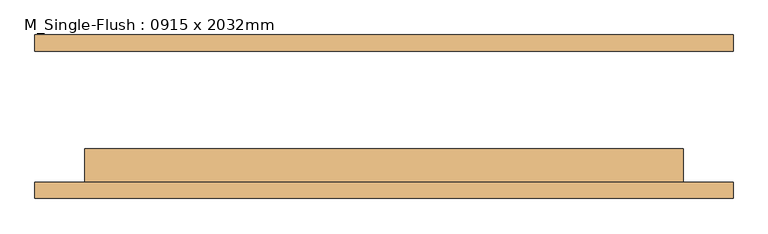
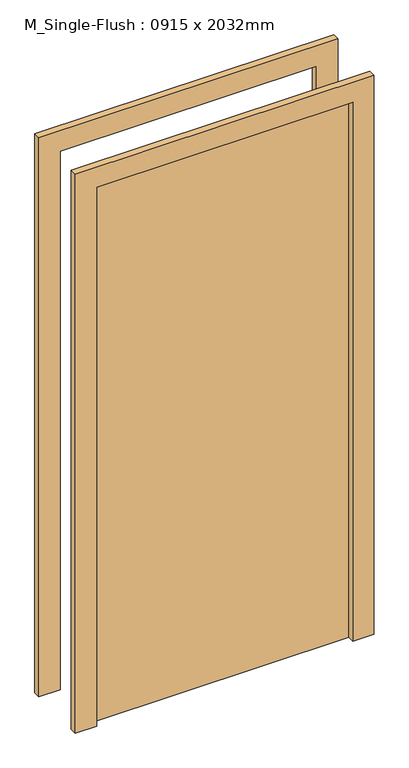
"""IFC4 building model written with IfcOpenShell, lengths in millimetres: door geometry, M_Single-Flush : 0915 x 2032mm."""

from ifc_helpers import new_model, si_unit, frame, origin, origin_with_axes, place, context, project, spatial, polyline, outline, extrude, source, transform, mapped, element, save


def m_single_flush_0915_x_2032mm_26613924(model_context):
    return source(origin(), model_context, "Body", "SweptSolid", [
        extrude(outline(polyline([(2108.0, -533.5), (0.0, -533.5), (0.0, -457.5), (2032.0, -457.5), (2032.0, 457.5), (0.0, 457.5), (0.0, 533.5), (2108.0, 533.5), (2108.0, -533.5)])), frame((0.0, -125.0, 0.0), z_axis=(0.0, 1.0, 0.0), x_axis=(0.0, 0.0, 1.0)), (0.0, 0.0, 1.0), 25.0),
        extrude(outline(polyline([(2108.0, 533.5), (2108.0, -533.5), (0.0, -533.5), (0.0, -457.5), (2032.0, -457.5), (2032.0, 457.5), (0.0, 457.5), (0.0, 533.5), (2108.0, 533.5)])), frame((0.0, 100.0, 0.0), z_axis=(0.0, 1.0, 0.0), x_axis=(0.0, 0.0, 1.0)), (0.0, 0.0, 1.0), 25.0),
        extrude(outline(polyline([(457.5, -49.0), (457.5, -100.0), (-457.5, -100.0), (-457.5, -49.0), (457.5, -49.0)])), origin_with_axes(), (0.0, 0.0, 1.0), 2032.0),
    ])


if __name__ == "__main__":
    model = new_model("IFC4")
    model_context = context("Model", 3, world=origin())
    ifc_project = project(units=[si_unit("LENGTHUNIT", "METRE", prefix="MILLI")], contexts=[model_context])
    site = spatial("IfcSite", under=ifc_project)
    building = spatial("IfcBuilding", under=site)
    placement = place(None, origin())
    m_single_flush_0915_x_2032mm_shape = m_single_flush_0915_x_2032mm_26613924(model_context)
    element("IfcDoor", 1, ObjectType="M_Single-Flush : 0915 x 2032mm", at=placement, inside=building, context=model_context, shape_type="MappedRepresentation", body=[
        mapped(m_single_flush_0915_x_2032mm_shape, transform((0.0, 0.0, 0.0), x_axis=(1.0, 0.0, 0.0), y_axis=(0.0, 1.0, 0.0), z_axis=(0.0, 0.0, 1.0))),
    ])
    save(model, "model.ifc")

# Revit data of these elements
# Type "M_Single-Flush : 0915 x 2032mm"
#   Type Mark = "20"
#   Thickness = 0' - 2.00787"
#   Height = 6' - 8"
#   Trim Projection Ext = 0' - 0.98425"
#   Trim Projection Int = 0' - 0.98425"
#   Trim Width = 0' - 2.99213"
#   Width = 3' - 0.02362"
#   Door Material = Door - Panel
#   Frame Material = Door - Frame
#   Function = (empty or 0)
#   Wall Closure = (empty or 0)
# Element 1 (IfcDoor, "M_Single-Flush : 0915 x 2032mm")
#   Materials on its faces: "Door - Frame", "Door - Panel"
# Materials
#   "Door - Panel": class "Wood", colour RGB 114 82 51, transparency 0
#   "Door - Frame": colour RGB 153 76 43, transparency 0
